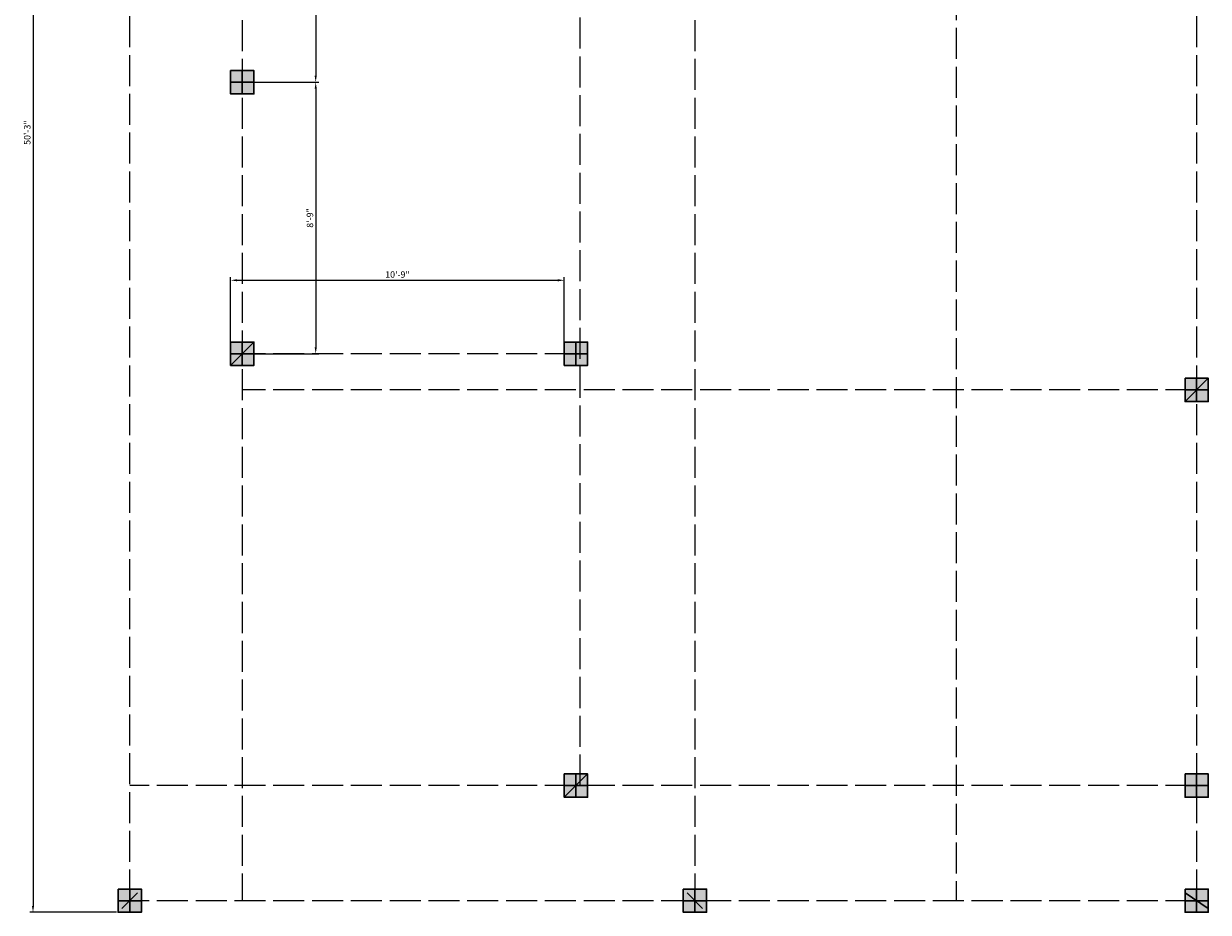
# Model space of a CAD drawing. Units: inches. Extents: x 2163 to 7246, y 928 to 2098.
# Tile 8 of 15: x 2733 to 3191, y 1411 to 1754. Entities that reach past the tile are written whole.
import ezdxf

# ---------------------------------------------------------------- set-up
doc = ezdxf.new("R2010")
doc.units = ezdxf.units.IN
doc.linetypes.add('ACAD_ISO02W100', pattern=[15, 12, -3])
for name, color, linetype, lineweight in [('A-ANNO-DIMS', 4, 'Continuous', 18), ('A-COLS', 41, 'Continuous', 30), ('A-GRID', 1, 'ACAD_ISO02W100', 18)]:
    doc.layers.add(name, color=color, linetype=linetype, lineweight=lineweight)
doc.layers.add('A-COLS-PATT', color=51, linetype='Continuous', lineweight=9, true_color=0xf8f6b0)
doc.styles.get("Standard").update_dxf_attribs({"font": 'arial.ttf'})
doc.dimstyles.new('ISO-25', dxfattribs={"dimtxt": 2.5, "dimasz": 2.5, "dimexe": 1.25, "dimexo": 0.625, "dimtad": 1, "dimdec": 0, "dimlunit": 3, "dimtxsty": 'Standard', "dimcen": 2.5, "dimadec": 0, "dimazin": 0, "dimtfac": 1, "dimtdec": 0, "dimtmove": 0, "dimatfit": 3, "dimfxl": 1, "dimarcsym": 0})

# ---------------------------------------------------------------- blocks, each defined once
blk = doc.blocks.new('COL-9X9-CENTERED')
for p, q in [((4.5, 9), (4.5, 0)), ((0, 4.5), (9, 4.5))]:
    blk.add_line(p, q)
blk.add_lwpolyline([(0, 9), (9, 9), (9, 0), (0, 0)], close=True)
blk = doc.blocks.new('*D80')
at = {"layer": 'A-ANNO-DIMS', "color": 0, "lineweight": -2, "transparency": 16777216}
for p, q in [((2768.6, 2013.57), (2735.07, 2013.57)), ((2736.32, 2011.07), (2736.32, 1413.07)), ((2768.6, 1410.57), (2735.07, 1410.57))]:
    blk.add_line(p, q, dxfattribs=at)
at = {"layer": 'A-ANNO-DIMS', "color": 0, "transparency": 16777216}
for points in [[(2735.91, 2011.07), (2736.74, 2011.07), (2736.32, 2013.57)], [(2735.91, 1413.07), (2736.74, 1413.07), (2736.32, 1410.57)]]:
    blk.add_solid(points, dxfattribs=at)
at = {"layer": 'Defpoints', "color": 0, "transparency": 16777216}
for p in [(2769.22, 2013.57), (2736.32, 1410.57), (2769.22, 1410.57)]:
    blk.add_point(p, dxfattribs=at)
at = {"layer": 'A-ANNO-DIMS', "color": 0, "transparency": 16777216, "insert": (2734.42, 1712.07), "char_height": 2.5, "attachment_point": 5, "rotation": 90}
blk.add_mtext('50\'-3"', dxfattribs=at)
blk = doc.blocks.new('*D83')
at = {"layer": 'A-ANNO-DIMS', "color": 0, "lineweight": -2, "transparency": 16777216}
for p, q in [((2812.72, 1622.7), (2812.72, 1656.22)), ((2815.22, 1654.97), (2939.22, 1654.97)), ((2941.72, 1622.7), (2941.72, 1656.22))]:
    blk.add_line(p, q, dxfattribs=at)
at = {"layer": 'A-ANNO-DIMS', "color": 0, "transparency": 16777216}
for points in [[(2815.22, 1655.39), (2815.22, 1654.56), (2812.72, 1654.97)], [(2939.22, 1655.39), (2939.22, 1654.56), (2941.72, 1654.97)]]:
    blk.add_solid(points, dxfattribs=at)
at = {"layer": 'Defpoints', "color": 0, "transparency": 16777216}
for p in [(2941.72, 1654.97), (2812.72, 1622.07), (2941.72, 1622.07)]:
    blk.add_point(p, dxfattribs=at)
at = {"layer": 'A-ANNO-DIMS', "color": 0, "transparency": 16777216, "insert": (2877.22, 1656.87), "char_height": 2.5, "attachment_point": 5}
blk.add_mtext('10\'-9"', dxfattribs=at)
blk = doc.blocks.new('*D91')
at = {"layer": 'A-ANNO-DIMS', "color": 0, "lineweight": -2, "transparency": 16777216}
for p, q in [((2813.35, 1812.57), (2846.87, 1812.57)), ((2845.62, 1810.07), (2845.62, 1734.07)), ((2813.35, 1731.57), (2846.87, 1731.57))]:
    blk.add_line(p, q, dxfattribs=at)
at = {"layer": 'A-ANNO-DIMS', "color": 0, "transparency": 16777216}
for points in [[(2845.21, 1810.07), (2846.04, 1810.07), (2845.62, 1812.57)], [(2845.21, 1734.07), (2846.04, 1734.07), (2845.62, 1731.57)]]:
    blk.add_solid(points, dxfattribs=at)
at = {"layer": 'Defpoints', "color": 0, "transparency": 16777216}
for p in [(2812.72, 1812.57), (2812.72, 1731.57), (2845.62, 1731.57)]:
    blk.add_point(p, dxfattribs=at)
at = {"layer": 'A-ANNO-DIMS', "color": 0, "transparency": 16777216, "insert": (2843.72, 1772.07), "char_height": 2.5, "attachment_point": 5, "rotation": 90}
blk.add_mtext('6\'-9"', dxfattribs=at)
blk = doc.blocks.new('*D92')
at = {"layer": 'A-ANNO-DIMS', "color": 0, "lineweight": -2, "transparency": 16777216}
for p, q in [((2813.35, 1731.57), (2846.87, 1731.57)), ((2845.62, 1729.07), (2845.62, 1629.07)), ((2813.35, 1626.57), (2846.87, 1626.57))]:
    blk.add_line(p, q, dxfattribs=at)
at = {"layer": 'A-ANNO-DIMS', "color": 0, "transparency": 16777216}
for points in [[(2845.21, 1729.07), (2846.04, 1729.07), (2845.62, 1731.57)], [(2845.21, 1629.07), (2846.04, 1629.07), (2845.62, 1626.57)]]:
    blk.add_solid(points, dxfattribs=at)
at = {"layer": 'Defpoints', "color": 0, "transparency": 16777216}
for p in [(2812.72, 1731.57), (2812.72, 1626.57), (2845.62, 1626.57)]:
    blk.add_point(p, dxfattribs=at)
at = {"layer": 'A-ANNO-DIMS', "color": 0, "transparency": 16777216, "insert": (2843.72, 1679.07), "char_height": 2.5, "attachment_point": 5, "rotation": 90}
blk.add_mtext('8\'-9"', dxfattribs=at)

msp = doc.modelspace()

# ---------------------------------------------------------------- hatches: boundary and pattern name
at = {"layer": 'A-COLS-PATT'}
h = msp.add_hatch(color=256, dxfattribs=at)
h.dxf.hatch_style = 1
h.paths.add_polyline_path([(2778.22, 2009.07), (2773.72, 2009.07), (2773.72, 2004.57), (2778.22, 2004.57)])
h.paths.add_polyline_path([(2778.22, 2013.57), (2773.72, 2013.57), (2773.72, 2009.07), (2778.22, 2009.07)])
h.paths.add_polyline_path([(2773.72, 2013.57), (2769.22, 2013.57), (2769.22, 2009.07), (2773.72, 2009.07)])
h.paths.add_polyline_path([(2773.72, 2009.07), (2769.22, 2009.07), (2769.22, 2004.57), (2773.72, 2004.57)])
h.paths.add_polyline_path([(2817.22, 1965.57), (2812.72, 1965.57), (2812.72, 1961.07), (2817.22, 1961.07)])
h.paths.add_polyline_path([(2817.22, 1970.07), (2812.72, 1970.07), (2817.22, 1965.57)])
h.paths.add_polyline_path([(2821.72, 1965.57), (2817.22, 1965.57), (2821.72, 1961.07)], flags=17)
h.paths.add_polyline_path([(2817.22, 1965.57), (2817.22, 1961.07), (2821.72, 1961.07)], flags=17)
h.paths.add_polyline_path([(2821.72, 1970.07), (2817.22, 1970.07), (2817.22, 1965.57), (2821.72, 1965.57)])
h.paths.add_polyline_path([(2812.72, 1970.07), (2812.72, 1965.57), (2817.22, 1965.57)], flags=17)
h.paths.add_polyline_path([(2992.22, 1970.07), (2987.72, 1970.07), (2987.72, 1965.57), (2992.22, 1965.57)])
h.paths.add_polyline_path([(2996.72, 1970.07), (2992.22, 1970.07), (2992.22, 1965.57), (2996.72, 1965.57)])
h.paths.add_polyline_path([(2996.72, 1965.57), (2992.22, 1965.57), (2992.22, 1961.07), (2996.72, 1961.07)])
h.paths.add_polyline_path([(2992.22, 1965.57), (2987.72, 1965.57), (2987.72, 1961.07), (2992.22, 1961.07)])
h.paths.add_polyline_path([(3097.72, 2012.07), (3093.22, 2012.07), (3093.22, 2009.07), (3097.72, 2009.07)])
h.paths.add_polyline_path([(3093.22, 2012.07), (3088.72, 2012.07), (3091.72, 2009.07), (3093.22, 2009.07)])
h.paths.add_polyline_path([(3091.72, 2009.07), (3088.72, 2009.07), (3088.72, 2007.57), (3093.22, 2007.57)])
h.paths.add_polyline_path([(3088.72, 2012.07), (3088.72, 2009.07), (3091.72, 2009.07)])
h.paths.add_polyline_path([(3097.72, 2009.07), (3093.22, 2009.07), (3093.22, 2007.57), (3097.72, 2007.57)])
h.paths.add_polyline_path([(3093.22, 2009.07), (3091.72, 2009.07), (3093.22, 2007.57)], flags=17)
h.paths.add_polyline_path([(3093.22, 2007.57), (3088.72, 2007.57), (3088.72, 2003.07), (3093.22, 2003.07)])
h.paths.add_polyline_path([(3093.22, 2007.57), (3093.22, 2003.07), (3097.72, 2003.07)])
h.paths.add_polyline_path([(3097.72, 2007.57), (3093.22, 2007.57), (3097.72, 2003.07)], flags=17)
h.paths.add_polyline_path([(3186.22, 2012.07), (3181.72, 2012.07), (3181.72, 2009.07), (3186.22, 2009.07)])
h.paths.add_polyline_path([(3190.72, 2012.07), (3186.22, 2012.07), (3186.22, 2009.07), (3187.72, 2009.07)])
h.paths.add_polyline_path([(3190.72, 2012.07), (3187.72, 2009.07), (3190.72, 2009.07)], flags=17)
h.paths.add_polyline_path([(3190.72, 2009.07), (3187.72, 2009.07), (3186.22, 2007.57), (3190.72, 2007.57)])
h.paths.add_polyline_path([(3187.72, 2009.07), (3186.22, 2009.07), (3186.22, 2007.57)], flags=17)
h.paths.add_polyline_path([(3186.22, 2009.07), (3181.72, 2009.07), (3181.72, 2007.57), (3186.22, 2007.57)])
h.paths.add_polyline_path([(3186.22, 2007.57), (3181.72, 2007.57), (3181.72, 2003.07)], flags=17)
h.paths.add_polyline_path([(3186.22, 2007.57), (3181.72, 2003.07), (3186.22, 2003.07)], flags=17)
h.paths.add_polyline_path([(3190.72, 2007.57), (3186.22, 2007.57), (3186.22, 2003.07), (3190.72, 2003.07)])
h.paths.add_polyline_path([(2817.22, 1812.57), (2812.72, 1812.57), (2812.72, 1808.07), (2817.22, 1808.07)])
h.paths.add_polyline_path([(2817.22, 1817.07), (2812.72, 1817.07), (2812.72, 1812.57), (2817.22, 1812.57)])
h.paths.add_polyline_path([(2821.72, 1817.07), (2817.22, 1817.07), (2817.22, 1812.57), (2821.72, 1812.57)])
h.paths.add_polyline_path([(2821.72, 1812.57), (2817.22, 1812.57), (2817.22, 1808.07), (2821.72, 1808.07)])
h.paths.add_polyline_path([(2821.72, 1736.07), (2817.22, 1736.07), (2817.22, 1731.57), (2821.72, 1731.57)])
h.paths.add_polyline_path([(2817.22, 1736.07), (2812.72, 1736.07), (2812.72, 1731.57), (2817.22, 1731.57)])
h.paths.add_polyline_path([(2817.22, 1731.57), (2812.72, 1731.57), (2812.72, 1727.07), (2817.22, 1727.07)])
h.paths.add_polyline_path([(2821.72, 1731.57), (2817.22, 1731.57), (2817.22, 1727.07), (2821.72, 1727.07)])
h.paths.add_polyline_path([(2992.22, 1765.57), (2987.72, 1761.07), (2992.22, 1761.07)], flags=17)
h.paths.add_polyline_path([(2992.22, 1765.57), (2987.72, 1765.57), (2987.72, 1761.07)])
h.paths.add_polyline_path([(2992.22, 1770.07), (2987.72, 1770.07), (2987.72, 1765.57), (2992.22, 1765.57)])
h.paths.add_polyline_path([(2996.72, 1770.07), (2992.22, 1770.07), (2992.22, 1765.57)])
h.paths.add_polyline_path([(2996.72, 1770.07), (2992.22, 1765.57), (2996.72, 1765.57)], flags=17)
h.paths.add_polyline_path([(2996.72, 1765.57), (2992.22, 1765.57), (2992.22, 1761.07), (2996.72, 1761.07)])
h.paths.add_polyline_path([(3097.72, 1770.07), (3093.22, 1770.07), (3093.22, 1765.57), (3097.72, 1765.57)])
h.paths.add_polyline_path([(3093.22, 1770.07), (3088.72, 1770.07), (3088.72, 1765.57), (3093.22, 1765.57)])
h.paths.add_polyline_path([(3093.22, 1765.57), (3088.72, 1765.57), (3088.72, 1761.07), (3093.22, 1761.07)])
h.paths.add_polyline_path([(3097.72, 1765.57), (3093.22, 1765.57), (3093.22, 1761.07), (3097.72, 1761.07)])
h.paths.add_polyline_path([(3186.22, 1770.07), (3181.72, 1770.07), (3181.72, 1765.57), (3186.22, 1765.57)])
h.paths.add_polyline_path([(3190.72, 1770.07), (3186.22, 1770.07), (3186.22, 1765.57), (3190.72, 1765.57)])
h.paths.add_polyline_path([(3190.72, 1765.57), (3186.22, 1765.57), (3186.22, 1761.07), (3190.72, 1761.07)])
h.paths.add_polyline_path([(3186.22, 1765.57), (3181.72, 1765.57), (3181.72, 1761.07), (3186.22, 1761.07)])
h.paths.add_polyline_path([(2946.22, 1626.57), (2941.72, 1626.57), (2941.72, 1622.07), (2946.22, 1622.07)])
h.paths.add_polyline_path([(2946.22, 1631.07), (2941.72, 1631.07), (2941.72, 1626.57), (2946.22, 1626.57)])
h.paths.add_polyline_path([(2950.72, 1631.07), (2947.91, 1631.07), (2947.91, 1626.57), (2950.72, 1626.57)])
h.paths.add_polyline_path([(2947.91, 1631.07), (2946.22, 1631.07), (2946.22, 1626.57), (2947.91, 1626.57)])
h.paths.add_polyline_path([(2947.91, 1626.57), (2946.22, 1626.57), (2946.22, 1622.07), (2947.91, 1622.07)])
h.paths.add_polyline_path([(2950.72, 1626.57), (2947.91, 1626.57), (2947.91, 1622.07), (2950.72, 1622.07)])
h.paths.add_polyline_path([(2821.72, 1626.57), (2817.22, 1626.57), (2817.22, 1622.07), (2821.72, 1622.07)])
h.paths.add_polyline_path([(2821.72, 1631.07), (2817.22, 1626.57), (2821.72, 1626.57)])
h.paths.add_polyline_path([(2821.72, 1631.07), (2817.22, 1631.07), (2817.22, 1626.57)], flags=17)
h.paths.add_polyline_path([(2817.22, 1631.07), (2812.72, 1631.07), (2812.72, 1626.57), (2817.22, 1626.57)])
h.paths.add_polyline_path([(2817.22, 1626.57), (2812.72, 1626.57), (2812.72, 1622.07)], flags=17)
h.paths.add_polyline_path([(2817.22, 1626.57), (2812.72, 1622.07), (2817.22, 1622.07)])
h.paths.add_polyline_path([(3190.72, 1612.57), (3186.22, 1612.57), (3186.22, 1608.07), (3190.72, 1608.07)])
h.paths.add_polyline_path([(3186.22, 1612.57), (3181.72, 1608.07), (3186.22, 1608.07)], flags=17)
h.paths.add_polyline_path([(3186.22, 1612.57), (3181.72, 1612.57), (3181.72, 1608.07)], flags=17)
h.paths.add_polyline_path([(3186.22, 1617.07), (3181.72, 1617.07), (3181.72, 1612.57), (3186.22, 1612.57)])
h.paths.add_polyline_path([(3190.72, 1617.07), (3186.22, 1617.07), (3186.22, 1612.57)], flags=17)
h.paths.add_polyline_path([(3190.72, 1617.07), (3186.22, 1612.57), (3190.72, 1612.57)], flags=17)
h.paths.add_polyline_path([(2950.72, 1459.57), (2946.22, 1459.57), (2946.22, 1455.07), (2950.72, 1455.07)])
h.paths.add_polyline_path([(2946.22, 1459.57), (2941.72, 1455.07), (2946.22, 1455.07)])
h.paths.add_polyline_path([(2946.22, 1459.57), (2941.72, 1459.57), (2941.72, 1455.07)])
h.paths.add_polyline_path([(2946.22, 1464.07), (2941.72, 1464.07), (2941.72, 1459.57), (2946.22, 1459.57)])
h.paths.add_polyline_path([(2947.91, 1464.07), (2946.22, 1464.07), (2946.22, 1459.57), (2947.91, 1461.26)])
h.paths.add_polyline_path([(2950.72, 1464.07), (2947.91, 1464.07), (2947.91, 1461.26)])
h.paths.add_polyline_path([(2950.72, 1464.07), (2947.91, 1461.26), (2947.91, 1459.57), (2950.72, 1459.57)])
h.paths.add_polyline_path([(2950.72, 1459.57), (2947.91, 1459.57), (2946.22, 1459.57), (2946.22, 1455.07), (2950.72, 1455.07)], flags=17)
h.paths.add_polyline_path([(2947.91, 1461.26), (2946.22, 1459.57), (2947.91, 1459.57)], flags=17)
h.paths.add_polyline_path([(2773.72, 1415.07), (2769.22, 1415.07), (2769.22, 1410.57), (2773.72, 1410.57)])
h.paths.add_polyline_path([(2778.22, 1415.07), (2773.72, 1415.07), (2773.72, 1410.57), (2778.22, 1410.57)])
h.paths.add_polyline_path([(2778.22, 1419.57), (2773.72, 1419.57), (2773.72, 1415.07), (2778.22, 1415.07)])
h.paths.add_polyline_path([(2773.72, 1419.57), (2769.22, 1419.57), (2769.22, 1415.07), (2773.72, 1415.07)])
h.paths.add_polyline_path([(2992.22, 1415.07), (2987.72, 1415.07), (2987.72, 1410.57), (2992.22, 1410.57)])
h.paths.add_polyline_path([(2992.22, 1419.57), (2987.72, 1419.57), (2987.72, 1415.07), (2992.22, 1415.07)])
h.paths.add_polyline_path([(2996.72, 1419.57), (2992.22, 1419.57), (2992.22, 1415.07), (2996.72, 1415.07)])
h.paths.add_polyline_path([(2992.22, 1415.07), (2992.22, 1410.57), (2996.72, 1410.57), (2996.72, 1415.07)])
h = msp.add_hatch(color=256, dxfattribs=at)
h.dxf.hatch_style = 1
h.paths.add_polyline_path([(2950.72, 1459.57), (2946.22, 1459.57), (2946.22, 1455.07), (2950.72, 1455.07)])
h.paths.add_polyline_path([(3186.22, 1415.07), (3181.72, 1415.07), (3181.72, 1410.57), (3186.22, 1410.57)])
h.paths.add_polyline_path([(3186.22, 1415.07), (3186.22, 1410.57), (3190.72, 1410.57), (3190.72, 1412.07)])
h.paths.add_polyline_path([(3190.72, 1415.07), (3186.22, 1415.07), (3190.72, 1412.07)])
h.paths.add_polyline_path([(3190.72, 1419.57), (3186.22, 1419.57), (3186.22, 1415.07), (3190.72, 1415.07)])
h.paths.add_polyline_path([(3186.22, 1419.57), (3181.72, 1419.57), (3181.72, 1418.07), (3186.22, 1415.07)])
h.paths.add_polyline_path([(3181.72, 1418.07), (3181.72, 1415.07), (3186.22, 1415.07)], flags=17)
h.paths.add_polyline_path([(3186.22, 1459.57), (3181.72, 1459.57), (3181.72, 1455.07), (3186.22, 1455.07)])
h.paths.add_polyline_path([(3186.22, 1464.07), (3181.72, 1464.07), (3181.72, 1459.57), (3186.22, 1459.57)])
h.paths.add_polyline_path([(3190.72, 1464.07), (3186.22, 1464.07), (3186.22, 1459.57), (3190.72, 1459.57)])
h.paths.add_polyline_path([(3190.72, 1459.57), (3186.22, 1459.57), (3186.22, 1455.07), (3190.72, 1455.07)])

# ---------------------------------------------------------------- linework, layer by layer
at = {"layer": 'A-COLS'}
for p, q in [((2821.72, 1631.07), (2812.72, 1622.07)), ((3181.72, 1608.07), (3190.72, 1617.07)), ((3190.72, 1617.07), (3190.72, 1617.07)), ((2950.72, 1464.07), (2941.72, 1455.07)), ((2776.72, 1418.07), (2770.72, 1412.07)), ((2995.22, 1412.07), (2989.22, 1418.07)), ((3181.72, 1418.07), (3190.72, 1412.07))]:
    msp.add_line(p, q, dxfattribs=at)
at = {"layer": 'A-GRID'}
for p, q in [((3186.22, 2012.07), (3186.22, 1415.07)), ((2773.72, 1415.07), (2773.72, 2009.07)), ((3093.22, 2007.57), (3093.22, 1415.07)), ((2817.22, 1965.57), (2817.22, 1415.07)), ((2947.91, 1459.57), (2947.91, 1965.57)), ((2992.22, 1965.57), (2992.22, 1415.07)), ((2946.22, 1626.57), (2812.72, 1626.57)), ((3186.22, 1612.57), (2817.22, 1612.57)), ((3186.22, 1459.57), (2773.72, 1459.57)), ((2992.22, 1415.07), (2992.22, 1419.57)), ((3186.22, 1415.07), (2773.72, 1415.07))]:
    msp.add_line(p, q, dxfattribs=at)

# ---------------------------------------------------------------- block references
at = {"layer": 'A-COLS'}
for p in [(2812.72, 1727.07), (2812.72, 1622.07), (2941.72, 1622.07), (3181.72, 1608.07), (2941.72, 1455.07), (3181.72, 1455.07), (2769.22, 1410.57), (2987.72, 1410.57), (3181.72, 1410.57)]:
    msp.add_blockref('COL-9X9-CENTERED', p, dxfattribs=at)

# ---------------------------------------------------------------- dimensions: what is measured, and where the dimension line sits
at = {"layer": 'A-ANNO-DIMS'}
for base, p1, p2, angle, picture, middle in [((2736.32, 1410.57), (2769.22, 2013.57), (2769.22, 1410.57), 90, '*D80', (2734.42, 1712.07)), ((2845.62, 1731.57), (2812.72, 1812.57), (2812.72, 1731.57), 270, '*D91', (2843.72, 1772.07)), ((2845.62, 1626.57), (2812.72, 1731.57), (2812.72, 1626.57), 270, '*D92', (2843.72, 1679.07))]:
    dim = msp.add_linear_dim(base=base, p1=p1, p2=p2, angle=angle, dimstyle='ISO-25', override={"dimdec": 1, "dimlfac": 1, "dimrnd": 0, "dimzin": 1, "dimdsep": 46, "dimlunit": 4, "dimfrac": 2}, dxfattribs=at)
    dim.commit()
    dim.dimension.update_dxf_attribs({"geometry": picture, "text_midpoint": middle})
dim = msp.add_linear_dim(base=(2941.72, 1654.97), p1=(2812.72, 1622.07), p2=(2941.72, 1622.07), dimstyle='ISO-25', override={"dimdec": 1, "dimlfac": 1, "dimrnd": 0, "dimzin": 1, "dimdsep": 46, "dimlunit": 4, "dimfrac": 2}, dxfattribs=at)
dim.commit()
dim.dimension.update_dxf_attribs({"geometry": '*D83', "text_midpoint": (2877.22, 1656.87)})

doc.saveas('drawing.dxf')
